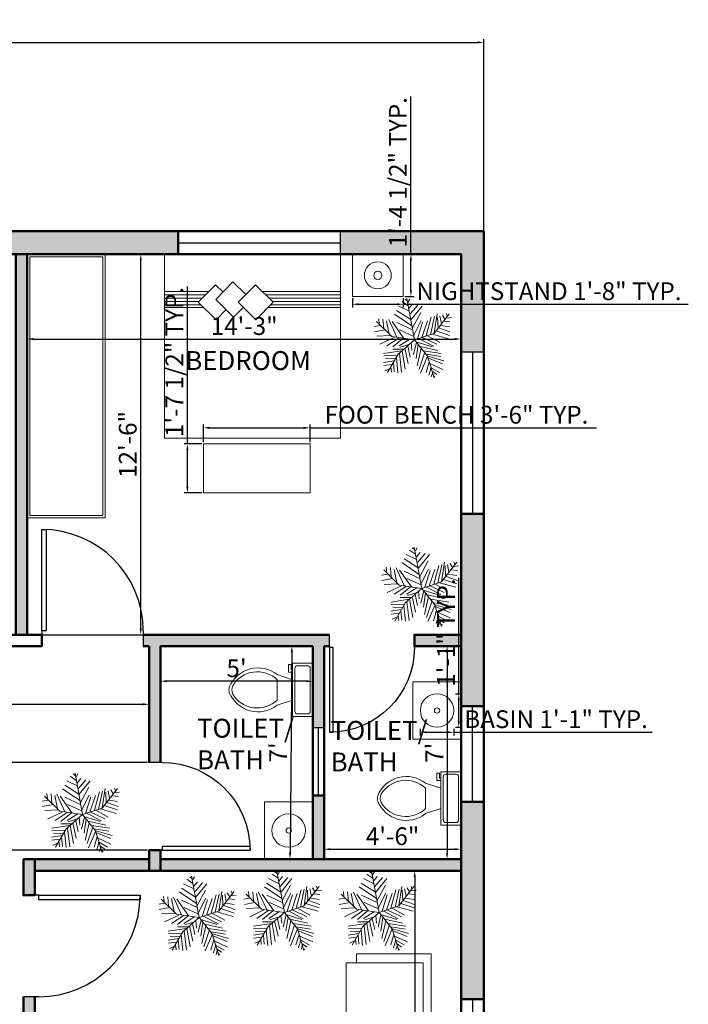
# Model space of a CAD drawing. Units: inches. Extents: x 1647 to 2354, y 1705 to 2321.
# Tile 4 of 4: x 2085 to 2349, y 1919 to 2307. Entities that reach past the tile are written whole.
import ezdxf

# ---------------------------------------------------------------- set-up
doc = ezdxf.new("R2010")
doc.units = ezdxf.units.IN
for name, color, linetype, lineweight in [('A-ANNO-DIMS', 130, 'Continuous', 18), ('A-AREA-IDEN', 7, 'Continuous', 25), ('A-FLOR-FIXT', 52, 'Continuous', 18), ('A-WALL-PATT', 84, 'Continuous', 13), ('door', 142, 'Continuous', 25), ('fur', 52, 'Continuous', 18), ('tree', 92, 'Continuous', 13), ('wall', 84, 'Continuous', 50), ('window', 242, 'Continuous', 25)]:
    doc.layers.add(name, color=color, linetype=linetype, lineweight=lineweight)
doc.styles.get("Standard").update_dxf_attribs({"font": 'arial.ttf'})
doc.dimstyles.new('ISO-25', dxfattribs={"dimtxt": 7, "dimasz": 2.5, "dimexe": 1.25, "dimexo": 0.625, "dimtad": 1, "dimdec": 0, "dimlunit": 4, "dimtxsty": 'Standard', "dimcen": 2.5, "dimadec": 0, "dimazin": 0, "dimtfac": 1, "dimtdec": 0, "dimtmove": 0, "dimatfit": 3, "dimfxl": 1, "dimarcsym": 0})

# ---------------------------------------------------------------- blocks, each defined once
blk = doc.blocks.new('*U2')
for p, q in [((0, 0), (0, -6)), ((40, 0), (40, -6))]:
    blk.add_line(p, q)
blk.add_lwpolyline([(0, 0), (0, 40), (1.75, 40), (1.75, 0)], close=True)
blk.add_arc((0, 0), 40, 0, 90)
blk = doc.blocks.new('*U4')
for p, q in [((9.5, -6), (9.5, -2)), ((-10, -8.5), (-8, -8.5)), ((-10, -9.5), (-10, -8.5)), ((-7, -9.5), (-10, -9.5)), ((-8, -8.5), (-8, -8)), ((-7, -8), (-7, -9.5)), ((-4, -8), (-6, -14)), ((4, -8), (6, -14)), ((4, -14), (-4, -14))]:
    blk.add_line(p, q)
blk.add_lwpolyline([(10.5, -8), (10.5, 0), (-10.5, 0), (-10.5, -8)], close=True)
for points in [[(-9.5, -2), (-9.5, -6)], [(8.5, -1), (-8.5, -1)], [(-8.5, -7), (8.5, -7)]]:
    blk.add_lwpolyline(points)
for centre, radius, start, end in [((-8.62, -1.88), 0.884, 81.8699, 188.1301), ((8.62, -1.88), 0.884, 351.8699, 98.1301), ((-8.62, -6.12), 0.884, 171.8699, 278.1301), ((8.62, -6.12), 0.884, 261.8699, 8.1301), ((3.52, -21.58), 12.17, 141.4691, 247.9714), ((4.2, -21.82), 11.33, 136.3677, 238.9468), ((-3.52, -21.58), 12.17, 292.0284, 38.5307), ((-4.2, -21.82), 11.33, 301.053, 43.6321), ((0, -27.88), 4, 245.7318, 294.2682), ((0, -29), 4, 254.8605, 285.1395)]:
    blk.add_arc(centre, radius, start, end)
blk = doc.blocks.new('*U6')
for p, q in [((-10.186, 53.64), (-13.084, 55.962)), ((0, 0), (-10.5, 57)), ((-9.099, 51.782), (-6.563, 55.962)), ((-7.288, 39.707), (-21.778, 46.673)), ((-8.737, 47.138), (-17.069, 52.711)), ((-7.65, 43.423), (-2.578, 49.46)), ((-5.839, 35.992), (4.667, 48.067)), ((-5.114, 27.632), (10.463, 46.673)), ((-48.585, 21.131), (-49.309, 29.026)), ((-43.513, 28.561), (-42.427, 15.558)), ((-35.544, 28.097), (-24.314, 3.947)), ((-3.665, 19.273), (-27.574, 35.527)), ((-5.114, 28.097), (-24.676, 40.636)), ((-2.941, 16.486), (8.652, 37.85)), ((16.259, 5.805), (23.142, 31.348)), ((22.055, 7.198), (27.489, 32.277)), ((27, 9), (48, 36)), ((27.127, 9.056), (31.112, 35.992)), ((31.836, 30.883), (32.561, 16.486)), ((35.096, 32.741), (37.27, 22.524)), ((38.719, 34.134), (41.979, 28.561)), ((43.791, 29.954), (51.036, 30.883)), ((44.153, 36.456), (45.239, 32.741)), ((-47.498, 19.737), (-55.83, 18.344)), ((-40.615, 13.7), (-55.105, 10.913)), ((-31.5, 4.5), (-52.5, 25.5)), ((-38.442, 26.239), (-34.819, 7.663)), ((-14.533, 2.09), (-30.834, 25.31)), ((-24.314, 23.917), (-2.941, 13.7)), ((-20.691, 13.7), (-1.129, 4.876)), ((-1.129, 6.734), (9.014, 26.704)), ((3.942, 1.625), (11.187, 24.381)), ((10.101, 3.483), (17.708, 26.239)), ((33.285, 16.486), (48.862, 10.913)), ((36.183, 19.737), (48.137, 17.88)), ((40.53, 25.775), (48.862, 24.846)), ((-33.37, 6.269), (-52.207, 5.34)), ((-28.299, 3.483), (-47.86, -5.805)), ((-21.416, 3.018), (-38.079, -8.128)), ((0, 0), (-31.5, 4.5)), ((-15.982, 2.09), (-30.11, -9.521)), ((0, 0), (-22.5, -19.5)), ((-6.563, 1.161), (-21.416, -8.128)), ((0, 0), (27, 9)), ((0, 0), (18, -22.5)), ((6.478, 1.625), (26.04, -8.592)), ((11.187, 3.483), (30.749, -5.805)), ((18.07, 5.805), (35.096, -3.483)), ((24.229, 7.663), (46.688, 1.625)), ((29.662, 12.307), (48.137, 6.269)), ((-15.257, -12.772), (-30.11, -12.772)), ((-6.563, -5.805), (-19.967, -9.985)), ((-13.446, -11.378), (-8.737, -32.741)), ((-9.461, -8.592), (-6.201, -23.453)), ((-4.752, -3.483), (-3.665, -14.629)), ((2.493, -3.019), (-1.491, -20.202)), ((1.769, -2.555), (24.229, -9.521)), ((5.029, -6.27), (2.131, -25.775)), ((9.014, -11.378), (3.58, -35.992)), ((7.565, -9.056), (32.198, -14.629)), ((-17.431, -15.094), (-42.789, -18.809)), ((-24.314, -21.596), (-42.427, -22.06)), ((-26.849, -26.24), (-40.253, -25.775)), ((-22.5, -19.5), (-37.5, -45)), ((-25.038, -23.918), (-22.865, -45.281)), ((-20.691, -18.345), (-17.793, -44.352)), ((-17.069, -15.094), (-12.721, -40.172)), ((14.085, -16.951), (6.478, -40.172)), ((18.07, -22.524), (8.289, -45.745)), ((12.274, -15.094), (36.907, -18.809)), ((16.259, -19.738), (36.183, -22.989)), ((18, -22.5), (27, -52.5)), ((18.433, -22.524), (40.53, -29.026)), ((19.157, -25.311), (38.719, -33.206)), ((-28.299, -29.026), (-42.789, -31.348)), ((-30.834, -34.135), (-42.427, -35.528)), ((-34.457, -39.708), (-40.978, -42.494)), ((-32.646, -36.921), (-31.921, -44.352)), ((-29.023, -30.884), (-27.936, -43.887)), ((20.244, -30.419), (15.897, -44.816)), ((22.78, -37.85), (19.519, -48.532)), ((21.331, -32.741), (39.081, -40.636)), ((22.78, -38.314), (34.372, -44.816)), ((24.591, -45.745), (23.142, -50.854)), ((24.591, -43.423), (30.749, -47.603)), ((26.764, -49.925), (28.213, -50.854))]:
    blk.add_line(p, q)
blk = doc.blocks.new('*D11')
at = {"layer": 'A-ANNO-DIMS', "color": 0, "lineweight": -2, "transparency": 16777216}
for p, q in [((2088.13, 2213.61), (2088.13, 2179.52)), ((2259.13, 2213.61), (2259.13, 2179.52)), ((2090.63, 2180.77), (2256.63, 2180.77))]:
    blk.add_line(p, q, dxfattribs=at)
at = {"layer": 'A-ANNO-DIMS', "color": 0, "transparency": 16777216}
for points in [[(2090.63, 2181.19), (2090.63, 2180.35), (2088.13, 2180.77)], [(2256.63, 2181.19), (2256.63, 2180.35), (2259.13, 2180.77)]]:
    blk.add_solid(points, dxfattribs=at)
at = {"layer": 'Defpoints', "color": 0, "transparency": 16777216}
for p in [(2088.13, 2214.23), (2259.13, 2214.23), (2259.13, 2180.77)]:
    blk.add_point(p, dxfattribs=at)
at = {"layer": 'A-ANNO-DIMS', "color": 0, "transparency": 16777216, "insert": (2173.63, 2184.97), "char_height": 7, "attachment_point": 5}
blk.add_mtext('14\'-3"', dxfattribs=at)
blk = doc.blocks.new('*D12')
at = {"layer": 'A-ANNO-DIMS', "color": 0, "lineweight": -2, "transparency": 16777216}
for p, q in [((2088.76, 2214.23), (2134.1, 2214.23)), ((2132.85, 2066.73), (2132.85, 2211.73)), ((2088.76, 2064.23), (2134.1, 2064.23))]:
    blk.add_line(p, q, dxfattribs=at)
at = {"layer": 'A-ANNO-DIMS', "color": 0, "transparency": 16777216}
for points in [[(2132.43, 2211.73), (2133.27, 2211.73), (2132.85, 2214.23)], [(2132.43, 2066.73), (2133.27, 2066.73), (2132.85, 2064.23)]]:
    blk.add_solid(points, dxfattribs=at)
at = {"layer": 'Defpoints', "color": 0, "transparency": 16777216}
for p in [(2088.13, 2214.23), (2132.85, 2214.23), (2088.13, 2064.23)]:
    blk.add_point(p, dxfattribs=at)
at = {"layer": 'A-ANNO-DIMS', "color": 0, "transparency": 16777216, "insert": (2128.65, 2139.23), "char_height": 7, "attachment_point": 5, "rotation": 90}
blk.add_mtext('12\'-6"', dxfattribs=at)
blk = doc.blocks.new('*D18')
at = {"layer": 'A-ANNO-DIMS', "color": 0, "lineweight": -2, "transparency": 16777216}
for p, q in [((2258.51, 1971.23), (2239.61, 1971.23)), ((2240.86, 1968.73), (2240.86, 1814.73)), ((2258.51, 1812.23), (2239.61, 1812.23))]:
    blk.add_line(p, q, dxfattribs=at)
at = {"layer": 'A-ANNO-DIMS', "color": 0, "transparency": 16777216}
for points in [[(2240.44, 1968.73), (2241.28, 1968.73), (2240.86, 1971.23)], [(2240.44, 1814.73), (2241.28, 1814.73), (2240.86, 1812.23)]]:
    blk.add_solid(points, dxfattribs=at)
at = {"layer": 'Defpoints', "color": 0, "transparency": 16777216}
for p in [(2259.13, 1971.23), (2240.86, 1812.23), (2259.13, 1812.23)]:
    blk.add_point(p, dxfattribs=at)
at = {"layer": 'A-ANNO-DIMS', "color": 0, "transparency": 16777216, "insert": (2236.66, 1891.73), "char_height": 7, "attachment_point": 5, "rotation": 90}
blk.add_mtext('13\'-3"', dxfattribs=at)
blk = doc.blocks.new('*D19')
at = {"layer": 'A-ANNO-DIMS', "color": 0, "lineweight": -2, "transparency": 16777216}
for p, q in [((2140.63, 2059.11), (2140.63, 2044.68)), ((2200.63, 2059.11), (2200.63, 2044.68)), ((2198.13, 2045.93), (2143.13, 2045.93))]:
    blk.add_line(p, q, dxfattribs=at)
at = {"layer": 'A-ANNO-DIMS', "color": 0, "transparency": 16777216}
for points in [[(2143.13, 2046.34), (2143.13, 2045.51), (2140.63, 2045.93)], [(2198.13, 2046.34), (2198.13, 2045.51), (2200.63, 2045.93)]]:
    blk.add_solid(points, dxfattribs=at)
at = {"layer": 'Defpoints', "color": 0, "transparency": 16777216}
for p in [(2140.63, 2059.73), (2200.63, 2059.73), (2140.63, 2045.93)]:
    blk.add_point(p, dxfattribs=at)
at = {"layer": 'A-ANNO-DIMS', "color": 0, "transparency": 16777216, "insert": (2170.63, 2050.11), "char_height": 7, "attachment_point": 5}
blk.add_mtext("5'", dxfattribs=at)
blk = doc.blocks.new('*D20')
at = {"layer": 'A-ANNO-DIMS', "color": 0, "lineweight": -2, "transparency": 16777216}
for p, q in [((2200.01, 2059.74), (2191.19, 2059.82)), ((2192.42, 2057.31), (2191.71, 1978.31)), ((2199.26, 1975.74), (2190.44, 1975.82))]:
    blk.add_line(p, q, dxfattribs=at)
at = {"layer": 'A-ANNO-DIMS', "color": 0, "transparency": 16777216}
for points in [[(2192, 2057.31), (2192.84, 2057.3), (2192.44, 2059.81)], [(2191.29, 1978.31), (2192.13, 1978.3), (2191.69, 1975.81)]]:
    blk.add_solid(points, dxfattribs=at)
at = {"layer": 'Defpoints', "color": 0, "transparency": 16777216}
for p in [(2200.63, 2059.73), (2191.69, 1975.81), (2199.88, 1975.73)]:
    blk.add_point(p, dxfattribs=at)
at = {"layer": 'A-ANNO-DIMS', "color": 0, "transparency": 16777216, "insert": (2187.94, 2017.84), "char_height": 7, "attachment_point": 5, "rotation": 89.487}
blk.add_mtext("7'", dxfattribs=at)
blk = doc.blocks.new('*D21')
at = {"layer": 'A-ANNO-DIMS', "color": 0, "lineweight": -2, "transparency": 16777216}
for p, q in [((2205.13, 1976.36), (2205.13, 1980.96)), ((2207.63, 1979.71), (2256.63, 1979.71)), ((2259.13, 1976.36), (2259.13, 1980.96))]:
    blk.add_line(p, q, dxfattribs=at)
at = {"layer": 'A-ANNO-DIMS', "color": 0, "transparency": 16777216}
for points in [[(2207.63, 1980.12), (2207.63, 1979.29), (2205.13, 1979.71)], [(2256.63, 1980.12), (2256.63, 1979.29), (2259.13, 1979.71)]]:
    blk.add_solid(points, dxfattribs=at)
at = {"layer": 'Defpoints', "color": 0, "transparency": 16777216}
for p in [(2259.13, 1979.71), (2205.13, 1975.73), (2259.13, 1975.73)]:
    blk.add_point(p, dxfattribs=at)
at = {"layer": 'A-ANNO-DIMS', "color": 0, "transparency": 16777216, "insert": (2232.13, 1983.91), "char_height": 7, "attachment_point": 5}
blk.add_mtext('4\'-6"', dxfattribs=at)
blk = doc.blocks.new('*D22')
at = {"layer": 'A-ANNO-DIMS', "color": 0, "lineweight": -2, "transparency": 16777216}
for p, q in [((2258.51, 2059.73), (2252.36, 2059.73)), ((2253.61, 2057.23), (2253.61, 1978.23)), ((2258.51, 1975.73), (2252.36, 1975.73))]:
    blk.add_line(p, q, dxfattribs=at)
at = {"layer": 'A-ANNO-DIMS', "color": 0, "transparency": 16777216}
for points in [[(2253.2, 2057.23), (2254.03, 2057.23), (2253.61, 2059.73)], [(2253.2, 1978.23), (2254.03, 1978.23), (2253.61, 1975.73)]]:
    blk.add_solid(points, dxfattribs=at)
at = {"layer": 'Defpoints', "color": 0, "transparency": 16777216}
for p in [(2259.13, 2059.73), (2253.61, 1975.73), (2259.13, 1975.73)]:
    blk.add_point(p, dxfattribs=at)
at = {"layer": 'A-ANNO-DIMS', "color": 0, "transparency": 16777216, "insert": (2249.49, 2017.73), "char_height": 7, "attachment_point": 5, "rotation": 90}
blk.add_mtext("7'", dxfattribs=at)
blk = doc.blocks.new('*D23')
at = {"layer": 'A-ANNO-DIMS', "color": 0, "lineweight": -2, "transparency": 16777216}
for p, q in [((1909.63, 2059.11), (1909.63, 2035.57)), ((2136.13, 2059.11), (2136.13, 2035.57)), ((1912.13, 2036.82), (2133.63, 2036.82))]:
    blk.add_line(p, q, dxfattribs=at)
at = {"layer": 'A-ANNO-DIMS', "color": 0, "transparency": 16777216}
for points in [[(1912.13, 2037.24), (1912.13, 2036.41), (1909.63, 2036.82)], [(2133.63, 2037.24), (2133.63, 2036.41), (2136.13, 2036.82)]]:
    blk.add_solid(points, dxfattribs=at)
at = {"layer": 'Defpoints', "color": 0, "transparency": 16777216}
for p in [(1909.63, 2059.73), (2136.13, 2059.73), (2136.13, 2036.82)]:
    blk.add_point(p, dxfattribs=at)
at = {"layer": 'A-ANNO-DIMS', "color": 0, "transparency": 16777216, "insert": (2022.88, 2041.02), "char_height": 7, "attachment_point": 5}
blk.add_mtext('18\'-11"', dxfattribs=at)
blk = doc.blocks.new('*D24')
at = {"layer": 'A-ANNO-DIMS', "color": 0, "lineweight": -2, "transparency": 16777216}
for p, q in [((1728.13, 2223.86), (1728.13, 2298.93)), ((1730.63, 2297.68), (2265.63, 2297.68)), ((2268.13, 2223.86), (2268.13, 2298.93))]:
    blk.add_line(p, q, dxfattribs=at)
at = {"layer": 'A-ANNO-DIMS', "color": 0, "transparency": 16777216}
for points in [[(1730.63, 2298.09), (1730.63, 2297.26), (1728.13, 2297.68)], [(2265.63, 2298.09), (2265.63, 2297.26), (2268.13, 2297.68)]]:
    blk.add_solid(points, dxfattribs=at)
at = {"layer": 'Defpoints', "color": 0, "transparency": 16777216}
for p in [(2268.13, 2297.68), (1728.13, 2223.23), (2268.13, 2223.23)]:
    blk.add_point(p, dxfattribs=at)
at = {"layer": 'A-ANNO-DIMS', "color": 0, "transparency": 16777216, "insert": (1998.13, 2301.86), "char_height": 7, "attachment_point": 5}
blk.add_mtext("45'", dxfattribs=at)
blk = doc.blocks.new('WIN-WIDE-9IN-WALL')
blk.add_line((0, 4.5), (63.83, 4.5))
blk.add_lwpolyline([(0, 9), (63.83, 9), (63.83, 0), (0, 0)], close=True)
blk = doc.blocks.new('WIN-NARROW-9IN-WALL')
blk.add_line((4.5, 0), (4.5, 37.68))
blk.add_lwpolyline([(0, 37.68), (9, 37.68), (9, 0), (0, 0)], close=True)
blk = doc.blocks.new('WARDROBE-LONG')
for points in [[(0, 103.94), (30.72, 103.94), (30.72, 0), (0, 0)], [(1, 102.94), (29.72, 102.94), (29.72, 1), (1, 1)]]:
    blk.add_lwpolyline(points, close=True)
blk = doc.blocks.new('NIGHTSTAND-WITH-LAMP')
blk.add_lwpolyline([(0, 16.74), (20.08, 16.74), (20.08, 0), (0, 0)], close=True)
for radius in [5.31, 1.6]:
    blk.add_circle((10.04, 8.37), radius)
blk = doc.blocks.new('BED-PILLOW-AND-COVER-SET')
for p, q in [((0, 11.11), (17.43, 11.11)), ((0, 9.87), (16.21, 9.87)), ((0, 8.55), (14.92, 8.55)), ((38.64, 11.11), (69.38, 11.11)), ((39.89, 9.87), (69.38, 9.87)), ((41.22, 8.55), (69.38, 8.55)), ((0, 7.29), (13.67, 7.29)), ((0, 5.98), (14.28, 5.98)), ((0, 4.92), (15.36, 4.92)), ((31.01, 4.92), (31.05, 4.92)), ((40.88, 4.92), (69.38, 4.92)), ((41.93, 5.98), (69.38, 5.98)), ((42.51, 7.29), (69.38, 7.29))]:
    blk.add_line(p, q)
for points in [[(23.1, 10.95), (20.15, 13.86), (13.32, 6.93), (20.34, 0), (24.26, 3.97)], [(32.02, 9.99), (27.02, 14.92), (20.19, 7.99), (27.21, 1.06), (31.03, 4.93)]]:
    blk.add_lwpolyline(points)
blk.add_lwpolyline([(29.01, 6.93), (36.04, 0), (42.87, 6.93), (35.84, 13.86)], close=True)
blk = doc.blocks.new('BED-FOOT-BENCH')
blk.add_lwpolyline([(0, 19.36), (42.07, 19.36), (42.07, 0), (0, 0)], close=True)
blk = doc.blocks.new('LAV-BOWL-ROUND')
for radius in [6.59, 1.03]:
    blk.add_circle((6.59, 6.59), radius)
blk = doc.blocks.new('*D39')
at = {"layer": 'A-ANNO-DIMS', "color": 0, "lineweight": -2, "transparency": 16777216}
for p, q in [((2216.27, 2196.87), (2216.27, 2193.23)), ((2236.34, 2196.87), (2236.34, 2193.23)), ((2218.77, 2194.48), (2233.84, 2194.48)), ((2236.34, 2194.48), (2348.7, 2194.48))]:
    blk.add_line(p, q, dxfattribs=at)
at = {"layer": 'A-ANNO-DIMS', "color": 0, "transparency": 16777216}
for points in [[(2218.77, 2194.9), (2218.77, 2194.06), (2216.27, 2194.48)], [(2233.84, 2194.9), (2233.84, 2194.06), (2236.34, 2194.48)]]:
    blk.add_solid(points, dxfattribs=at)
at = {"layer": 'Defpoints', "color": 0, "transparency": 16777216}
for p in [(2216.27, 2197.49), (2236.34, 2197.49), (2236.34, 2194.48)]:
    blk.add_point(p, dxfattribs=at)
at = {"layer": 'A-ANNO-DIMS', "color": 0, "transparency": 16777216, "insert": (2293.77, 2198.72), "char_height": 7, "attachment_point": 5}
blk.add_mtext('NIGHTSTAND 1\'-8" TYP.', dxfattribs=at)
blk = doc.blocks.new('*D40')
at = {"layer": 'A-ANNO-DIMS', "color": 0, "lineweight": -2, "transparency": 16777216}
for p, q in [((2239.36, 2214.23), (2239.36, 2276.3)), ((2236.97, 2214.23), (2240.61, 2214.23)), ((2239.36, 2199.99), (2239.36, 2211.73)), ((2236.97, 2197.49), (2240.61, 2197.49))]:
    blk.add_line(p, q, dxfattribs=at)
at = {"layer": 'A-ANNO-DIMS', "color": 0, "transparency": 16777216}
for points in [[(2238.94, 2211.73), (2239.77, 2211.73), (2239.36, 2214.23)], [(2238.94, 2199.99), (2239.77, 2199.99), (2239.36, 2197.49)]]:
    blk.add_solid(points, dxfattribs=at)
at = {"layer": 'Defpoints', "color": 0, "transparency": 16777216}
for p in [(2236.34, 2214.23), (2239.36, 2214.23), (2236.34, 2197.49)]:
    blk.add_point(p, dxfattribs=at)
at = {"layer": 'A-ANNO-DIMS', "color": 0, "transparency": 16777216, "insert": (2235.11, 2246.52), "char_height": 7, "attachment_point": 5, "rotation": 90}
blk.add_mtext('1\'-4 1/2" TYP.', dxfattribs=at)
blk = doc.blocks.new('*D43')
at = {"layer": 'A-ANNO-DIMS', "color": 0, "lineweight": -2, "transparency": 16777216}
for p, q in [((2157.55, 2140.09), (2157.55, 2147.03)), ((2199.62, 2140.09), (2199.62, 2147.03)), ((2160.05, 2145.78), (2197.12, 2145.78)), ((2199.62, 2145.78), (2312.47, 2145.78))]:
    blk.add_line(p, q, dxfattribs=at)
at = {"layer": 'A-ANNO-DIMS', "color": 0, "transparency": 16777216}
for points in [[(2160.05, 2146.2), (2160.05, 2145.36), (2157.55, 2145.78)], [(2197.12, 2146.2), (2197.12, 2145.36), (2199.62, 2145.78)]]:
    blk.add_solid(points, dxfattribs=at)
at = {"layer": 'Defpoints', "color": 0, "transparency": 16777216}
for p in [(2199.62, 2145.78), (2157.55, 2139.47), (2199.62, 2139.47)]:
    blk.add_point(p, dxfattribs=at)
at = {"layer": 'A-ANNO-DIMS', "color": 0, "transparency": 16777216, "insert": (2257.3, 2150.03), "char_height": 7, "attachment_point": 5}
blk.add_mtext('FOOT BENCH 3\'-6" TYP.', dxfattribs=at)
blk = doc.blocks.new('*D44')
at = {"layer": 'A-ANNO-DIMS', "color": 0, "lineweight": -2, "transparency": 16777216}
for p, q in [((2151.24, 2139.47), (2151.24, 2201.54)), ((2156.93, 2139.47), (2149.99, 2139.47)), ((2151.24, 2122.61), (2151.24, 2136.97)), ((2156.93, 2120.11), (2149.99, 2120.11))]:
    blk.add_line(p, q, dxfattribs=at)
at = {"layer": 'A-ANNO-DIMS', "color": 0, "transparency": 16777216}
for points in [[(2150.83, 2136.97), (2151.66, 2136.97), (2151.24, 2139.47)], [(2150.83, 2122.61), (2151.66, 2122.61), (2151.24, 2120.11)]]:
    blk.add_solid(points, dxfattribs=at)
at = {"layer": 'Defpoints', "color": 0, "transparency": 16777216}
for p in [(2151.24, 2139.47), (2157.55, 2139.47), (2157.55, 2120.11)]:
    blk.add_point(p, dxfattribs=at)
at = {"layer": 'A-ANNO-DIMS', "color": 0, "transparency": 16777216, "insert": (2147, 2171.75), "char_height": 7, "attachment_point": 5, "rotation": 90}
blk.add_mtext('1\'-7 1/2" TYP.', dxfattribs=at)
blk = doc.blocks.new('*D51')
at = {"layer": 'A-ANNO-DIMS', "color": 0, "lineweight": -2, "transparency": 16777216}
for p, q in [((2243.06, 2027.16), (2243.06, 2024.56)), ((2245.56, 2025.81), (2253.74, 2025.81)), ((2256.24, 2027.16), (2256.24, 2024.56)), ((2256.24, 2025.81), (2334.41, 2025.81))]:
    blk.add_line(p, q, dxfattribs=at)
at = {"layer": 'A-ANNO-DIMS', "color": 0, "transparency": 16777216}
for points in [[(2245.56, 2026.23), (2245.56, 2025.39), (2243.06, 2025.81)], [(2253.74, 2026.23), (2253.74, 2025.39), (2256.24, 2025.81)]]:
    blk.add_solid(points, dxfattribs=at)
at = {"layer": 'Defpoints', "color": 0, "transparency": 16777216}
for p in [(2243.06, 2027.79), (2256.24, 2027.79), (2256.24, 2025.81)]:
    blk.add_point(p, dxfattribs=at)
at = {"layer": 'A-ANNO-DIMS', "color": 0, "transparency": 16777216, "insert": (2296.58, 2030.05), "char_height": 7, "attachment_point": 5}
blk.add_mtext('BASIN 1\'-1" TYP.', dxfattribs=at)
blk = doc.blocks.new('*D52')
at = {"layer": 'A-ANNO-DIMS', "color": 0, "lineweight": -2, "transparency": 16777216}
for p, q in [((2258.22, 2040.96), (2258.22, 2086.72)), ((2256.87, 2040.96), (2259.47, 2040.96)), ((2258.22, 2030.29), (2258.22, 2038.46)), ((2256.87, 2027.79), (2259.47, 2027.79))]:
    blk.add_line(p, q, dxfattribs=at)
at = {"layer": 'A-ANNO-DIMS', "color": 0, "transparency": 16777216}
for points in [[(2257.8, 2038.46), (2258.63, 2038.46), (2258.22, 2040.96)], [(2257.8, 2030.29), (2258.63, 2030.29), (2258.22, 2027.79)]]:
    blk.add_solid(points, dxfattribs=at)
at = {"layer": 'Defpoints', "color": 0, "transparency": 16777216}
for p in [(2256.24, 2040.96), (2258.22, 2040.96), (2256.24, 2027.79)]:
    blk.add_point(p, dxfattribs=at)
at = {"layer": 'A-ANNO-DIMS', "color": 0, "transparency": 16777216, "insert": (2254.08, 2065.09), "char_height": 7, "attachment_point": 5, "rotation": 90}
blk.add_mtext('1\'-1" TYP.', dxfattribs=at)
blk = doc.blocks.new('*D57')
at = {"layer": 'A-ANNO-DIMS', "color": 0, "lineweight": -2, "transparency": 16777216}
for p, q in [((2135.51, 2013.92), (1693.08, 2013.92)), ((1694.33, 2011.42), (1694.33, 1981.78)), ((2135.51, 1979.28), (1693.08, 1979.28)), ((1694.33, 1979.28), (1694.33, 1935.05))]:
    blk.add_line(p, q, dxfattribs=at)
at = {"layer": 'A-ANNO-DIMS', "color": 0, "transparency": 16777216}
for points in [[(1693.92, 2011.42), (1694.75, 2011.42), (1694.33, 2013.92)], [(1693.92, 1981.78), (1694.75, 1981.78), (1694.33, 1979.28)]]:
    blk.add_solid(points, dxfattribs=at)
at = {"layer": 'Defpoints', "color": 0, "transparency": 16777216}
for p in [(2136.13, 2013.92), (1694.33, 1979.28), (2136.13, 1979.28)]:
    blk.add_point(p, dxfattribs=at)
at = {"layer": 'A-ANNO-DIMS', "color": 0, "transparency": 16777216, "insert": (1690.09, 1955.92), "char_height": 7, "attachment_point": 5, "rotation": 90}
blk.add_mtext('2\'-10 1/2"', dxfattribs=at)

msp = doc.modelspace()

# ---------------------------------------------------------------- hatches: boundary and pattern name
at = {"layer": 'A-WALL-PATT'}
h = msp.add_hatch(color=256, dxfattribs=at)
h.dxf.hatch_style = 1
h.paths.add_polyline_path([(1737.13, 2214.23), (1778.6, 2214.23), (1778.6, 2223.23), (1728.13, 2223.23), (1728.13, 2080.92), (1737.13, 2080.92)])
h.paths.add_polyline_path([(1785.23, 1812.23), (1737.13, 1812.23), (1737.13, 1856.57), (1728.13, 1856.57), (1728.13, 1803.23), (1785.23, 1803.23)])
h.paths.add_polyline_path([(2020.88, 1812.23), (1967.48, 1812.23), (1967.48, 1803.23), (2020.88, 1803.23)])
h.paths.add_polyline_path([(2101.16, 1807.61), (2101.16, 1812.23), (2091.13, 1812.23), (2091.13, 1921.55), (2086.63, 1921.55), (2086.63, 1812.23), (2058.56, 1812.23), (2058.56, 1803.23), (2101.16, 1803.23)])
h.paths.add_polyline_path([(1929.8, 1812.23), (1909.63, 1812.23), (1909.63, 1848.23), (1909.63, 1917.89), (1905.13, 1917.89), (1905.13, 1812.23), (1882.72, 1812.23), (1849.06, 1812.23), (1849.06, 1803.23), (1929.8, 1803.23)])
h.paths.add_polyline_path([(2178.59, 1812.23), (2159.48, 1812.23), (2159.48, 1807.61), (2159.48, 1803.23), (2178.59, 1803.23)])
h.paths.add_polyline_path([(2268.13, 1856.83), (2259.13, 1856.83), (2259.13, 1815.23), (2259.13, 1812.23), (2242.42, 1812.23), (2242.42, 1803.23), (2268.13, 1803.23)])
h = msp.add_hatch(color=256, dxfattribs=at)
h.dxf.hatch_style = 1
h.paths.add_polyline_path([(1957.79, 2223.23), (1842.44, 2223.23), (1842.44, 2214.23), (1957.79, 2214.23)])
h.paths.add_polyline_path([(2147.66, 2223.23), (2021.62, 2223.23), (2021.62, 2214.23), (2147.66, 2214.23)])
h.paths.add_polyline_path([(2088.13, 2214.23), (2083.63, 2214.23), (2083.63, 2064.23), (2088.13, 2064.23)])
h.paths.add_polyline_path([(1909.63, 2214.23), (1905.13, 2214.23), (1905.13, 2059.73), (1909.63, 2059.73), (1909.63, 2064.23)])
h.paths.add_polyline_path([(1737.13, 2017.09), (1728.13, 2017.09), (1728.13, 1920.4), (1737.13, 1920.4)])
h.paths.add_polyline_path([(1905.13, 1975.23), (1737.13, 1975.23), (1737.13, 1970.73), (1905.13, 1970.73)])
h.paths.add_polyline_path([(1909.63, 2059.73), (1905.13, 2059.73), (1905.13, 1957.89), (1909.63, 1957.89)])
h.paths.add_polyline_path([(2036.41, 2064.23), (1909.63, 2064.23), (1909.63, 2059.73), (2036.41, 2059.73)])
h.paths.add_polyline_path([(2140.63, 1979.28), (2136.13, 1979.28), (2136.13, 1971.23), (2140.63, 1971.23)])
h.paths.add_polyline_path([(2136.13, 1975.73), (2091.13, 1975.73), (2091.13, 1971.23), (2136.13, 1971.23)])
h.paths.add_polyline_path([(2091.13, 1975.73), (2086.63, 1975.73), (2086.63, 1961.55), (2091.13, 1961.55)])
h.paths.add_polyline_path([(2259.13, 1975.73), (2140.63, 1975.73), (2140.63, 1971.23), (2259.13, 1971.23)])
h.paths.add_polyline_path([(2205.13, 2000.82), (2200.63, 2000.82), (2200.63, 1975.73), (2205.13, 1975.73)])
h.paths.add_polyline_path([(2268.13, 2111.84), (2259.13, 2111.84), (2259.13, 2036.03), (2268.13, 2036.03)])
h.paths.add_polyline_path([(2259.13, 2064.23), (2240.73, 2064.23), (2240.73, 2059.73), (2259.13, 2059.73)])
h.paths.add_polyline_path([(2268.13, 1998.35), (2259.13, 1998.35), (2259.13, 1989.23), (2259.13, 1920.66), (2268.13, 1920.66)])
h = msp.add_hatch(color=256, dxfattribs=at)
h.dxf.hatch_style = 1
h.paths.add_polyline_path([(2268.13, 2223.23), (2211.49, 2223.23), (2211.49, 2214.23), (2211.58, 2214.23), (2259.13, 2214.23), (2259.13, 2175.67), (2268.13, 2175.67)])
h.paths.add_polyline_path([(2207.29, 2064.23), (2133.85, 2064.23), (2133.85, 2059.73), (2136.13, 2059.73), (2136.13, 2013.92), (2140.63, 2013.92), (2140.63, 2059.73), (2200.63, 2059.73), (2200.63, 2027.71), (2205.13, 2027.71), (2205.13, 2059.73), (2207.29, 2059.73)])

# ---------------------------------------------------------------- linework, layer by layer
at = {"layer": 'A-FLOR-FIXT'}
msp.add_lwpolyline([(2259.13, 2023.04), (2240.17, 2023.04), (2240.17, 2045.71), (2259.13, 2045.71), (2259.13, 2036.03)], dxfattribs=at)
msp.add_lwpolyline([(2200.63, 1975.73), (2181.67, 1975.73), (2181.67, 1998.4), (2200.63, 1998.4)], close=True, dxfattribs=at)
at = {"layer": 'fur'}
for p, q in [((2217.9, 1934.94), (2217.9, 1938.45)), ((2217.9, 1938.45), (2247.32, 1938.45)), ((2247.32, 1938.45), (2247.32, 1844.07))]:
    msp.add_line(p, q, dxfattribs=at)
msp.add_lwpolyline([(2211.49, 2214.23), (2211.58, 2214.23), (2211.58, 2141.71), (2142.2, 2141.71), (2142.2, 2214.23), (2147.66, 2214.23)], dxfattribs=at)
msp.add_lwpolyline([(2244.21, 1934.94), (2213.88, 1934.94), (2213.88, 1847.66), (2244.21, 1847.66)], close=True, dxfattribs=at)
at = {"layer": 'wall'}
for p, q in [((1728.13, 2223.23), (2268.13, 2223.23)), ((2268.13, 2223.23), (2268.13, 1803.23)), ((2088.13, 2214.23), (2088.13, 2064.23)), ((2088.13, 2064.23), (2093.85, 2064.23)), ((2133.85, 2064.23), (2207.29, 2064.23)), ((2240.73, 2064.23), (2259.13, 2064.23)), ((2088.13, 2059.73), (2076.41, 2059.73)), ((2088.13, 2059.73), (2093.85, 2059.73)), ((2133.85, 2059.73), (2136.13, 2059.73)), ((2136.13, 2059.73), (2136.13, 2013.92)), ((2200.63, 2059.73), (2140.63, 2059.73)), ((2140.63, 2059.73), (2140.63, 2013.92)), ((2140.63, 2059.73), (2200.63, 2059.73)), ((2200.63, 1975.73), (2200.63, 2059.73)), ((2205.13, 1975.73), (2205.13, 2059.73)), ((2205.13, 2059.73), (2207.29, 2059.73)), ((2240.73, 2059.73), (2259.13, 2059.73)), ((2259.13, 2059.73), (2259.13, 1975.73)), ((2136.13, 1979.28), (2136.13, 1975.73)), ((2140.63, 1979.28), (2140.63, 1975.73)), ((2086.63, 1975.73), (2136.13, 1975.73)), ((2086.63, 1961.55), (2086.63, 1975.73)), ((2140.63, 1975.73), (2200.63, 1975.73)), ((2140.63, 1975.73), (2144.1, 1975.73)), ((2259.13, 1975.73), (2205.13, 1975.73)), ((2091.13, 1968.23), (2091.13, 1971.23)), ((2091.13, 1971.23), (2139.26, 1971.23)), ((2091.13, 1961.55), (2091.13, 1968.23)), ((2136.13, 1971.23), (2200.63, 1971.23)), ((2259.13, 1971.23), (2200.63, 1971.23)), ((2259.13, 1971.23), (2259.13, 1815.23)), ((2086.63, 1812.23), (2086.63, 1921.55)), ((2091.13, 1812.23), (2091.13, 1921.55))]:
    msp.add_line(p, q, dxfattribs=at)
for points in [[(2101.16, 1803.23), (1728.13, 1803.23), (1728.13, 2223.23), (2268.13, 2223.23), (2268.13, 1803.23), (2159.48, 1803.23)], [(2088.13, 2214.23), (2259.13, 2214.23), (2259.13, 2064.23)], [(2259.13, 2059.73), (2259.13, 1975.73)], [(2259.13, 1971.23), (2259.13, 1812.23), (2158.21, 1812.23)]]:
    msp.add_lwpolyline(points, dxfattribs=at)
for points in [[(2021.62, 2214.23), (2147.66, 2214.23), (2147.66, 2223.23), (2021.62, 2223.23)], [(2083.63, 2064.23), (2088.13, 2064.23), (2088.13, 2214.23), (2083.63, 2214.23)], [(2259.13, 2111.84), (2268.13, 2111.84), (2268.13, 2036.03), (2259.13, 2036.03)], [(2076.41, 2059.73), (2093.85, 2059.73), (2093.85, 2064.23), (2076.41, 2064.23)], [(2259.13, 2064.23), (2240.73, 2064.23), (2240.73, 2059.73), (2259.13, 2059.73)], [(2200.63, 2000.82), (2205.13, 2000.82), (2205.13, 1975.73), (2200.63, 1975.73)], [(2259.13, 1998.35), (2268.13, 1998.35), (2268.13, 1920.66), (2259.13, 1920.66)], [(2140.63, 1971.23), (2136.13, 1971.23), (2136.13, 1979.28), (2140.63, 1979.28)], [(2086.63, 1975.73), (2091.13, 1975.73), (2091.13, 1961.55), (2086.63, 1961.55)], [(2136.13, 1975.73), (2091.13, 1975.73), (2091.13, 1971.23), (2136.13, 1971.23)], [(2259.13, 1975.73), (2140.63, 1975.73), (2140.63, 1971.23), (2259.13, 1971.23)]]:
    msp.add_lwpolyline(points, close=True, dxfattribs=at)
at = {"layer": 'window'}
msp.add_line((2202.88, 2000.82), (2202.88, 2027.71), dxfattribs=at)
msp.add_lwpolyline([(2200.63, 2027.71), (2205.13, 2027.71), (2205.13, 2000.82), (2200.63, 2000.82)], close=True, dxfattribs=at)

# ---------------------------------------------------------------- block references
at = {"layer": 'A-FLOR-FIXT', "rotation": 270}
for p in [(2200.63, 2042.51), (2259.13, 1999.73)]:
    msp.add_blockref('*U4', p, dxfattribs=at)
at = {"layer": 'A-FLOR-FIXT'}
for p in [(2243.07, 2027.79), (2184.57, 1980.48)]:
    msp.add_blockref('LAV-BOWL-ROUND', p, dxfattribs=at)
at = {"layer": 'door'}
msp.add_blockref('*U2', (2093.85, 2065.73), dxfattribs=at)
for p, xscale, yscale, zscale, rotation in [((2207.29, 2059.22), -0.8359334157358912, 0.8359334157358912, 0.8359334157358912, 180), ((2141.33, 1979.28), -0.8659359851198896, 0.8659359851198896, 0.8659359851198896, 270)]:
    msp.add_blockref('*U2', p, dxfattribs=dict(at, xscale=xscale, yscale=yscale, zscale=zscale, rotation=rotation))
at = {"layer": 'door', "rotation": 270}
msp.add_blockref('*U2', (2092.63, 1961.55), dxfattribs=at)
at = {"layer": 'fur'}
for name, p in [('WARDROBE-LONG', (2088.13, 2110.29)), ('NIGHTSTAND-WITH-LAMP', (2216.27, 2197.49)), ('BED-PILLOW-AND-COVER-SET', (2142.2, 2188.34)), ('BED-FOOT-BENCH', (2157.55, 2120.11))]:
    msp.add_blockref(name, p, dxfattribs=at)
at = {"layer": 'tree', "xscale": 0.2858091163346259, "yscale": 0.2858091163346259, "zscale": 0.2858091163346259}
for p in [(2240.78, 2180.44), (2243.7, 2082.51), (2109.94, 1993.38), (2155.92, 1952.78), (2189.48, 1954.77), (2226.85, 1954.77)]:
    msp.add_blockref('*U6', p, dxfattribs=at)
at = {"layer": 'window'}
for name, p in [('WIN-WIDE-9IN-WALL', (2147.66, 2214.23)), ('WIN-NARROW-9IN-WALL', (2259.13, 1998.35))]:
    msp.add_blockref(name, p, dxfattribs=at)
at = {"layer": 'window', "rotation": 270.0000000000003}
for p in [(2259.13, 2175.67), (2259.13, 1920.66)]:
    msp.add_blockref('WIN-WIDE-9IN-WALL', p, dxfattribs=at)

# ---------------------------------------------------------------- texts
at = {"layer": 'A-AREA-IDEN', "char_height": 7.465, "attachment_point": 1}
for s, insert in [('BEDROOM', (2150.42, 2176.02)), ('TOILET/\\PBATH', (2155.06, 2031.12)), ('TOILET/\\PBATH', (2207.7, 2030.28))]:
    msp.add_mtext_dynamic_manual_height_columns(s, width=263.8302, gutter_width=37.32, heights=[0], dxfattribs=dict(at, insert=insert))

# ---------------------------------------------------------------- dimensions: what is measured, and where the dimension line sits
at = {"layer": 'A-ANNO-DIMS'}
for base, p1, p2, picture, middle in [((2268.13, 2297.68), (1728.13, 2223.23), (2268.13, 2223.23), '*D24', (1998.13, 2301.86)), ((2259.13, 2180.77), (2088.13, 2214.23), (2259.13, 2214.23), '*D11', (2173.63, 2184.97)), ((2136.13438186, 2036.82443058), (1909.63438186, 2059.73275818), (2136.13438186, 2059.73275818), '*D23', (2022.88438186, 2041.02344149)), ((2140.63, 2045.93), (2200.63, 2059.73), (2140.63, 2059.73), '*D19', (2170.63, 2050.11)), ((2259.13, 1979.71), (2205.13, 1975.73), (2259.13, 1975.73), '*D21', (2232.13, 1983.91))]:
    dim = msp.add_linear_dim(base=base, p1=p1, p2=p2, dimstyle='ISO-25', override={"dimclrd": 0, "dimclre": 0, "dimclrt": 0}, dxfattribs=at)
    dim.commit()
    dim.dimension.update_dxf_attribs({"geometry": picture, "text_midpoint": middle})
for base, p1, p2, picture, middle in [((2239.36, 2214.23), (2236.34, 2197.49), (2236.34, 2214.23), '*D40', (2235.11, 2246.52)), ((2151.24, 2139.47), (2157.55, 2120.11), (2157.55, 2139.47), '*D44', (2147, 2171.75)), ((2258.22, 2040.96), (2256.24, 2027.79), (2256.24, 2040.96), '*D52', (2254.08, 2065.09))]:
    dim = msp.add_linear_dim(base=base, p1=p1, p2=p2, angle=90, text='<> TYP.', dimstyle='ISO-25', override={"dimdec": 1, "dimlfac": 1, "dimrnd": 0, "dimzin": 1, "dimdsep": 46, "dimlunit": 4, "dimfrac": 2}, dxfattribs=at)
    dim.commit()
    dim.dimension.update_dxf_attribs({"geometry": picture, "text_midpoint": middle})
for base, p1, p2, override, picture, middle in [((2132.85, 2214.23), (2088.13, 2064.23), (2088.13, 2214.23), {"dimclrd": 0, "dimclre": 0, "dimclrt": 0}, '*D12', (2128.65, 2139.23)), ((2253.61, 1975.73), (2259.13, 2059.73), (2259.13, 1975.73), {"dimclrd": 0, "dimclre": 0, "dimclrt": 0}, '*D22', (2249.49, 2017.73)), ((1694.33, 1979.28), (2136.13, 2013.92), (2136.13, 1979.28), {"dimdec": 1, "dimlfac": 1, "dimrnd": 0, "dimzin": 1, "dimdsep": 46, "dimlunit": 4, "dimfrac": 2}, '*D57', (1690.09, 1955.92)), ((2240.86, 1812.23), (2259.13, 1971.23), (2259.13, 1812.23), {"dimclrd": 0, "dimclre": 0, "dimclrt": 0}, '*D18', (2236.66, 1891.73))]:
    dim = msp.add_linear_dim(base=base, p1=p1, p2=p2, angle=90, dimstyle='ISO-25', override=override, dxfattribs=at)
    dim.commit()
    dim.dimension.update_dxf_attribs({"geometry": picture, "text_midpoint": middle})
for base, p1, p2, text, picture, middle in [((2236.34, 2194.48), (2216.27, 2197.49), (2236.34, 2197.49), 'NIGHTSTAND <> TYP.', '*D39', (2293.77, 2198.72)), ((2199.62, 2145.78), (2157.55, 2139.47), (2199.62, 2139.47), 'FOOT BENCH <> TYP.', '*D43', (2257.3, 2150.03)), ((2256.24, 2025.81), (2243.06, 2027.79), (2256.24, 2027.79), 'BASIN <> TYP.', '*D51', (2296.58, 2030.05))]:
    dim = msp.add_linear_dim(base=base, p1=p1, p2=p2, text=text, dimstyle='ISO-25', override={"dimdec": 1, "dimlfac": 1, "dimrnd": 0, "dimzin": 1, "dimdsep": 46, "dimlunit": 4, "dimfrac": 2}, dxfattribs=at)
    dim.commit()
    dim.dimension.update_dxf_attribs({"geometry": picture, "text_midpoint": middle})
dim = msp.add_aligned_dim(p1=(2200.63, 2059.73), p2=(2199.88, 1975.73), distance=-8.19, dimstyle='ISO-25', override={"dimclrd": 0, "dimclre": 0, "dimclrt": 0}, dxfattribs=at)
dim.commit()
dim.dimension.update_dxf_attribs({"geometry": '*D20', "text_midpoint": (2187.94, 2017.84)})

doc.saveas('drawing.dxf')
